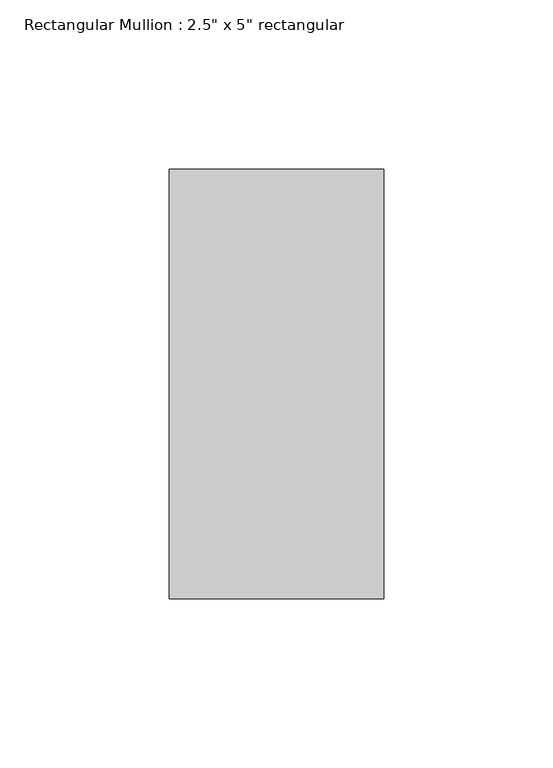
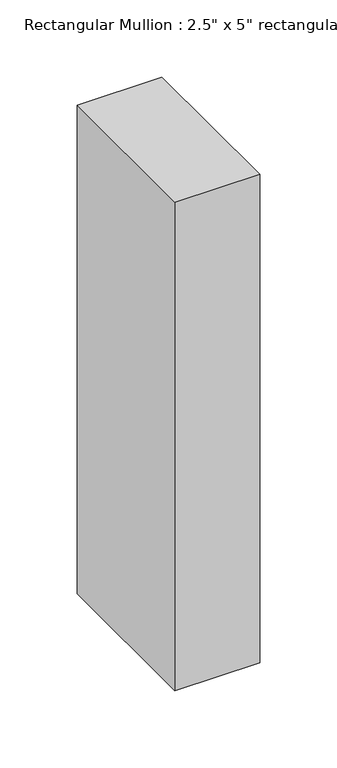
"""IFC4 building model written with IfcOpenShell, lengths in millimetres: member geometry."""

from ifc_helpers import new_model, si_unit, frame, origin, place, context, project, spatial, polyline, outline, extrude, source, transform, mapped, element, save


def member_dffdf235(model_context):
    return source(origin(), model_context, "Body", "SweptSolid", [
        extrude(outline(polyline([(0.0, 63.5), (0.0, -63.5), (-63.5, -63.5), (-63.5, 63.5), (0.0, 63.5)])), frame((0.0, 0.0, -387.35), z_axis=(0.0, 0.0, 1.0), x_axis=(1.0, 0.0, 0.0)), (0.0, 0.0, 1.0), 387.35),
    ])


if __name__ == "__main__":
    model = new_model("IFC4")
    model_context = context("Model", 3, world=origin())
    ifc_project = project(units=[si_unit("LENGTHUNIT", "METRE", prefix="MILLI")], contexts=[model_context])
    site = spatial("IfcSite", under=ifc_project)
    building = spatial("IfcBuilding", under=site)
    placement = place(None, origin())
    member_shape = member_dffdf235(model_context)
    element("IfcMember", 1, ObjectType="Rectangular Mullion : 2.5\" x 5\" rectangular", at=placement, inside=building, context=model_context, shape_type="MappedRepresentation", body=[
        mapped(member_shape, transform((0.0, 0.0, 0.0), x_axis=(1.0, 0.0, 0.0), y_axis=(0.0, 1.0, 0.0), z_axis=(0.0, 0.0, 1.0))),
    ])
    save(model, "model.ifc")

# Revit data of these elements
# Type "Rectangular Mullion : 2.5\" x 5\" rectangular"
#   built-in parameter 1007304 = 0.416667 (stored number, unit not read)
#   built-in parameter 1007301 = 0.104167 (stored number, unit not read)
#   built-in parameter 1007300 = 0.104167 (stored number, unit not read)
# Element 1 (IfcMember, "Rectangular Mullion : 2.5\" x 5\" rectangular")
#   Materials on its faces: "door colour"
# Materials
#   "door colour": class "Generic", colour RGB 120 120 120, transparency 0, Cost = 0
